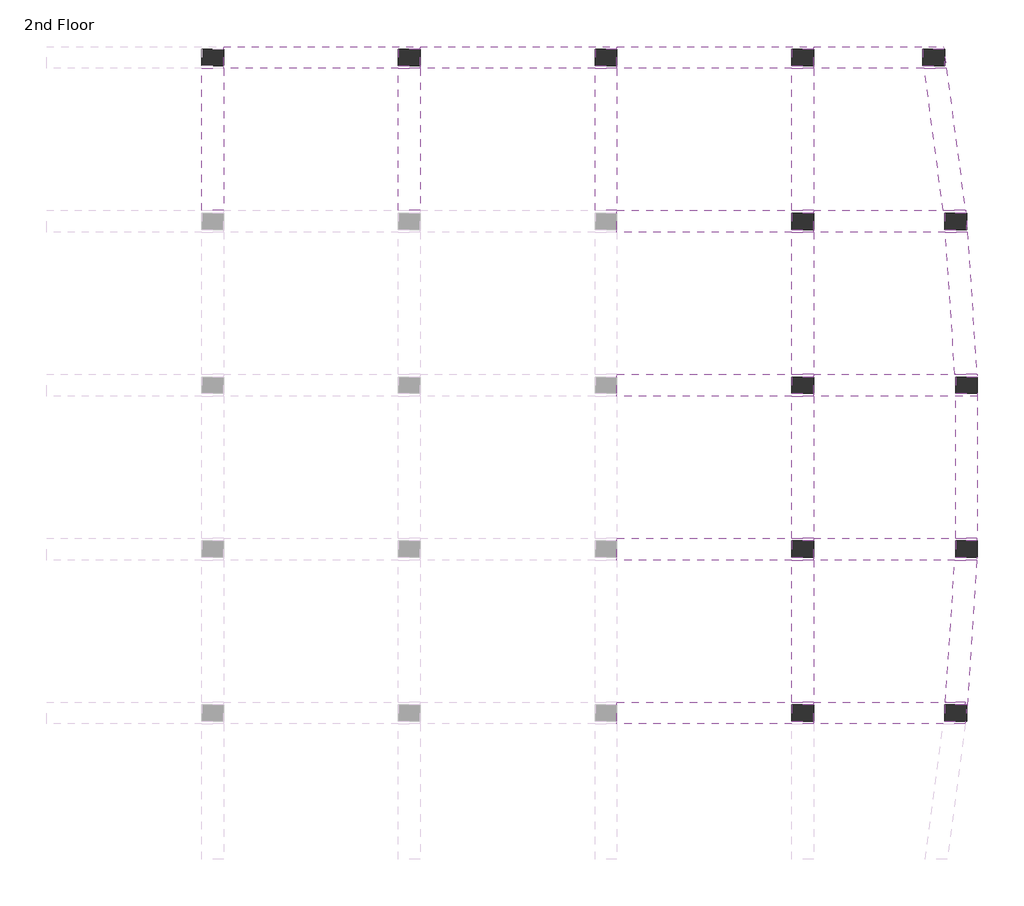
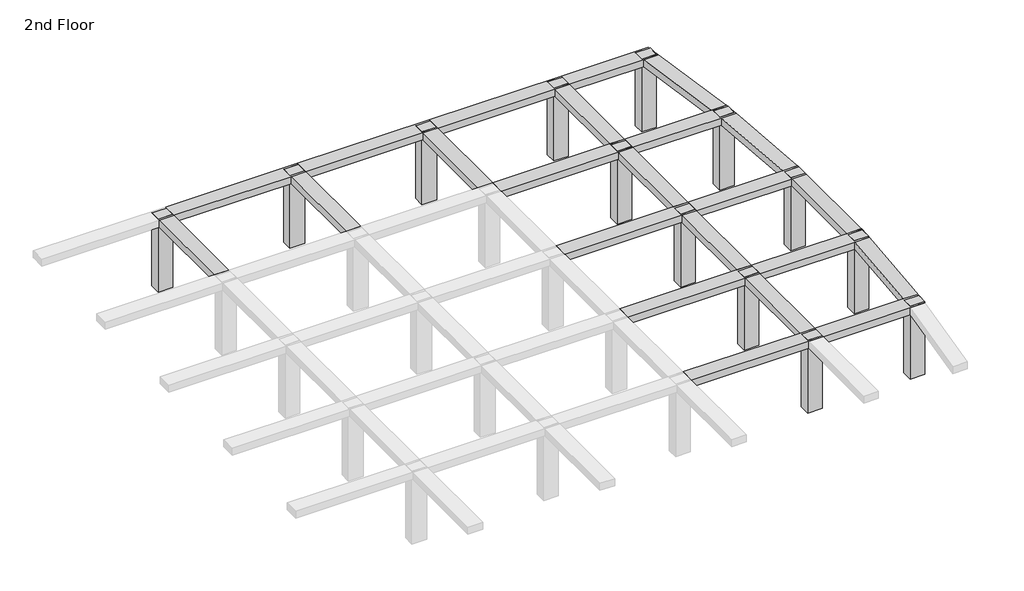
# One storey, part 3 of 3: 23 beams, 13 columns.
"""IFC4 building model written with IfcOpenShell, lengths in millimetres."""

from ifc_helpers import new_model, si_unit, frame, origin, place, context, project, spatial, polyline, outline, extrude, faceted_brep, element, save

model = new_model("IFC4")

# Units and contexts
model_context = context("Model", 3, world=origin())
ifc_project = project(units=[si_unit("LENGTHUNIT", "METRE", prefix="MILLI")], contexts=[model_context])

# Site, building, storey
site = spatial("IfcSite", under=ifc_project)
building = spatial("IfcBuilding", under=site)
storey = spatial("IfcBuildingStorey", under=building, Name="2nd Floor", Elevation=6400.8)

# Beams
placement = place(None, origin())
element("IfcBeam", 1, ObjectType="Concrete-Rectangular Beam : 2' x2'", at=placement, inside=storey, context=model_context, shape_type="Brep", body=[
    faceted_brep([(-160.074232, 1680.7831222, 9601.2), (-160.074232, 1604.5831222, 9601.2), (-160.074232, 1147.3831222, 9601.2), (-160.074232, 1071.1831222, 9601.2), (4716.725768, 1071.1831222, 9601.2), (5326.325768, 1071.1831222, 9601.2), (5326.325768, 1147.3831222, 9601.2), (4716.725768, 1147.3831222, 9601.2), (4716.725768, 1604.5831222, 9601.2), (5326.325768, 1604.5831222, 9601.2), (5326.325768, 1680.7831222, 9601.2), (4716.725768, 1680.7831222, 9601.2), (-160.074232, 1071.1831222, 9296.4), (4716.725768, 1071.1831222, 9296.4), (5326.325768, 1071.1831222, 9296.4), (-160.074232, 1147.3831222, 9296.4), (-160.074232, 1604.5831222, 9296.4), (-160.074232, 1680.7831222, 9296.4), (4716.725768, 1680.7831222, 9296.4), (5326.325768, 1680.7831222, 9296.4), (5326.325768, 1604.5831222, 9296.4), (4716.725768, 1604.5831222, 9296.4), (4716.725768, 1147.3831222, 9296.4), (5326.325768, 1147.3831222, 9296.4)], [[[0, 1, 2, 3, 4, 5, 6, 7, 8, 9, 10, 11]], [[3, 12, 13, 14, 5, 4]], [[12, 15, 16, 17, 18, 19, 20, 21, 22, 23, 14, 13]], [[10, 19, 18, 17, 0, 11]], [[3, 2, 1, 0, 17, 16, 15, 12]], [[5, 14, 23, 6]], [[22, 7, 6, 23]], [[7, 22, 21, 8]], [[8, 21, 20, 9]], [[19, 10, 9, 20]]]),
])
element("IfcBeam", 2, ObjectType="Concrete-Rectangular Beam : 2' x2'", at=placement, inside=storey, context=model_context, shape_type="Brep", body=[
    faceted_brep([(9555.2251658, 1680.7831222, 9601.2), (9003.0522312, 1680.7831222, 9601.2), (5326.325768, 1680.7831222, 9601.2), (5326.325768, 1604.5831222, 9601.2), (5326.325768, 1147.3831222, 9601.2), (5326.325768, 1071.1831222, 9601.2), (8940.2370643, 1071.1831222, 9601.2), (9555.2251658, 1071.1831222, 9601.2), (9555.2251658, 1147.3831222, 9601.2), (8983.5457827, 1147.3831222, 9601.2), (8983.5457827, 1604.5831222, 9601.2), (9555.2251658, 1604.5831222, 9601.2), (9555.2251658, 1071.1831222, 9296.4), (5326.325768, 1071.1831222, 9296.4), (8940.2370643, 1071.1831222, 9296.4), (5326.325768, 1147.3831222, 9296.4), (5326.325768, 1604.5831222, 9296.4), (5326.325768, 1680.7831222, 9296.4), (9003.0522312, 1680.7831222, 9296.4), (9555.2251658, 1680.7831222, 9296.4), (9555.2251658, 1604.5831222, 9296.4), (8983.5457827, 1604.5831222, 9296.4), (8983.5457827, 1147.3831222, 9296.4), (9555.2251658, 1147.3831222, 9296.4)], [[[0, 1, 2, 3, 4, 5, 6, 7, 8, 9, 10, 11]], [[12, 7, 6, 5, 13, 14]], [[12, 14, 13, 15, 16, 17, 18, 19, 20, 21, 22, 23]], [[0, 19, 18, 17, 2, 1]], [[7, 12, 23, 8]], [[5, 4, 3, 2, 17, 16, 15, 13]], [[22, 9, 8, 23]], [[9, 22, 21, 10]], [[10, 21, 20, 11]], [[19, 0, 11, 20]]]),
])
element("IfcBeam", 3, ObjectType="Concrete-Rectangular Beam : 2' x2'", at=placement, inside=storey, context=model_context, shape_type="Brep", body=[
    faceted_brep([(-160.074232, 6252.7831222, 9601.2), (-160.074232, 6176.5831222, 9601.2), (-160.074232, 5719.3831222, 9601.2), (-160.074232, 5643.1831222, 9601.2), (4716.725768, 5643.1831222, 9601.2), (5326.325768, 5643.1831222, 9601.2), (5326.325768, 5719.3831222, 9601.2), (4716.725768, 5719.3831222, 9601.2), (4716.725768, 6176.5831222, 9601.2), (5326.325768, 6176.5831222, 9601.2), (5326.325768, 6252.7831222, 9601.2), (4716.725768, 6252.7831222, 9601.2), (-160.074232, 5643.1831222, 9296.4), (4716.725768, 5643.1831222, 9296.4), (5326.325768, 5643.1831222, 9296.4), (-160.074232, 5719.3831222, 9296.4), (-160.074232, 6176.5831222, 9296.4), (-160.074232, 6252.7831222, 9296.4), (4716.725768, 6252.7831222, 9296.4), (5326.325768, 6252.7831222, 9296.4), (5326.325768, 6176.5831222, 9296.4), (4716.725768, 6176.5831222, 9296.4), (4716.725768, 5719.3831222, 9296.4), (5326.325768, 5719.3831222, 9296.4)], [[[0, 1, 2, 3, 4, 5, 6, 7, 8, 9, 10, 11]], [[3, 12, 13, 14, 5, 4]], [[12, 15, 16, 17, 18, 19, 20, 21, 22, 23, 14, 13]], [[10, 19, 18, 17, 0, 11]], [[3, 2, 1, 0, 17, 16, 15, 12]], [[5, 14, 23, 6]], [[22, 7, 6, 23]], [[7, 22, 21, 8]], [[8, 21, 20, 9]], [[19, 10, 9, 20]]]),
])
element("IfcBeam", 4, ObjectType="Concrete-Rectangular Beam : 2' x2'", at=placement, inside=storey, context=model_context, shape_type="Brep", body=[
    faceted_brep([(9876.2389574, 6252.7831222, 9601.2), (9286.1454059, 6252.7831222, 9601.2), (5326.325768, 6252.7831222, 9601.2), (5326.325768, 6176.5831222, 9601.2), (5326.325768, 5719.3831222, 9601.2), (5326.325768, 5643.1831222, 9601.2), (9265.305238, 5643.1831222, 9601.2), (9876.2389574, 5643.1831222, 9601.2), (9876.2389574, 5719.3831222, 9601.2), (9286.1454059, 5719.3831222, 9601.2), (9286.1454059, 6176.5831222, 9601.2), (9876.2389574, 6176.5831222, 9601.2), (9876.2389574, 5643.1831222, 9296.4), (5326.325768, 5643.1831222, 9296.4), (9265.305238, 5643.1831222, 9296.4), (5326.325768, 5719.3831222, 9296.4), (5326.325768, 6176.5831222, 9296.4), (5326.325768, 6252.7831222, 9296.4), (9286.1454059, 6252.7831222, 9296.4), (9876.2389574, 6252.7831222, 9296.4), (9876.2389574, 6176.5831222, 9296.4), (9286.1454059, 6176.5831222, 9296.4), (9286.1454059, 5719.3831222, 9296.4), (9876.2389574, 5719.3831222, 9296.4)], [[[0, 1, 2, 3, 4, 5, 6, 7, 8, 9, 10, 11]], [[12, 7, 6, 5, 13, 14]], [[12, 14, 13, 15, 16, 17, 18, 19, 20, 21, 22, 23]], [[0, 19, 18, 17, 2, 1]], [[7, 12, 23, 8]], [[5, 4, 3, 2, 17, 16, 15, 13]], [[22, 9, 8, 23]], [[9, 22, 21, 10]], [[10, 21, 20, 11]], [[19, 0, 11, 20]]]),
])
element("IfcBeam", 5, ObjectType="Concrete-Rectangular Beam : 2' x2'", at=placement, inside=storey, context=model_context, shape_type="Brep", body=[
    faceted_brep([(-160.074232, 10824.7831222, 9601.2), (-160.074232, 10748.5831222, 9601.2), (-160.074232, 10291.3831222, 9601.2), (-160.074232, 10215.1831222, 9601.2), (4716.725768, 10215.1831222, 9601.2), (5326.325768, 10215.1831222, 9601.2), (5326.325768, 10291.3831222, 9601.2), (4716.725768, 10291.3831222, 9601.2), (4716.725768, 10748.5831222, 9601.2), (5326.325768, 10748.5831222, 9601.2), (5326.325768, 10824.7831222, 9601.2), (4716.725768, 10824.7831222, 9601.2), (-160.074232, 10215.1831222, 9296.4), (4716.725768, 10215.1831222, 9296.4), (5326.325768, 10215.1831222, 9296.4), (-160.074232, 10291.3831222, 9296.4), (-160.074232, 10748.5831222, 9296.4), (-160.074232, 10824.7831222, 9296.4), (4716.725768, 10824.7831222, 9296.4), (5326.325768, 10824.7831222, 9296.4), (5326.325768, 10748.5831222, 9296.4), (4716.725768, 10748.5831222, 9296.4), (4716.725768, 10291.3831222, 9296.4), (5326.325768, 10291.3831222, 9296.4)], [[[0, 1, 2, 3, 4, 5, 6, 7, 8, 9, 10, 11]], [[3, 12, 13, 14, 5, 4]], [[12, 15, 16, 17, 18, 19, 20, 21, 22, 23, 14, 13]], [[10, 19, 18, 17, 0, 11]], [[3, 2, 1, 0, 17, 16, 15, 12]], [[5, 14, 23, 6]], [[22, 7, 6, 23]], [[7, 22, 21, 8]], [[8, 21, 20, 9]], [[19, 10, 9, 20]]]),
])
element("IfcBeam", 6, ObjectType="Concrete-Rectangular Beam : 2' x2'", at=placement, inside=storey, context=model_context, shape_type="Brep", body=[
    faceted_brep([(9895.7454059, 10824.7831222, 9601.2), (9876.2389574, 10824.7831222, 9601.2), (9265.305238, 10824.7831222, 9601.2), (5326.325768, 10824.7831222, 9601.2), (5326.325768, 10748.5831222, 9601.2), (5326.325768, 10291.3831222, 9601.2), (5326.325768, 10215.1831222, 9601.2), (9895.7454059, 10215.1831222, 9601.2), (9895.7454059, 10291.3831222, 9601.2), (9286.1454059, 10291.3831222, 9601.2), (9286.1454059, 10748.5831222, 9601.2), (9895.7454059, 10748.5831222, 9601.2), (9895.7454059, 10215.1831222, 9296.4), (5326.325768, 10215.1831222, 9296.4), (5326.325768, 10291.3831222, 9296.4), (5326.325768, 10748.5831222, 9296.4), (5326.325768, 10824.7831222, 9296.4), (9265.305238, 10824.7831222, 9296.4), (9876.2389574, 10824.7831222, 9296.4), (9895.7454059, 10824.7831222, 9296.4), (9895.7454059, 10748.5831222, 9296.4), (9286.1454059, 10748.5831222, 9296.4), (9286.1454059, 10291.3831222, 9296.4), (9895.7454059, 10291.3831222, 9296.4)], [[[0, 1, 2, 3, 4, 5, 6, 7, 8, 9, 10, 11]], [[12, 7, 6, 13]], [[12, 13, 14, 15, 16, 17, 18, 19, 20, 21, 22, 23]], [[0, 19, 18, 17, 16, 3, 2, 1]], [[7, 12, 23, 8]], [[6, 5, 4, 3, 16, 15, 14, 13]], [[22, 9, 8, 23]], [[9, 22, 21, 10]], [[10, 21, 20, 11]], [[19, 0, 11, 20]]]),
])
element("IfcBeam", 7, ObjectType="Concrete-Rectangular Beam : 2' x2'", at=placement, inside=storey, context=model_context, shape_type="Brep", body=[
    faceted_brep([(-160.074232, 15396.7831222, 9601.2), (-160.074232, 15320.5831222, 9601.2), (-160.074232, 14863.3831222, 9601.2), (-160.074232, 14787.1831222, 9601.2), (4716.725768, 14787.1831222, 9601.2), (5326.325768, 14787.1831222, 9601.2), (5326.325768, 14863.3831222, 9601.2), (4716.725768, 14863.3831222, 9601.2), (4716.725768, 15320.5831222, 9601.2), (5326.325768, 15320.5831222, 9601.2), (5326.325768, 15396.7831222, 9601.2), (4716.725768, 15396.7831222, 9601.2), (-160.074232, 14787.1831222, 9296.4), (4716.725768, 14787.1831222, 9296.4), (5326.325768, 14787.1831222, 9296.4), (-160.074232, 14863.3831222, 9296.4), (-160.074232, 15320.5831222, 9296.4), (-160.074232, 15396.7831222, 9296.4), (4716.725768, 15396.7831222, 9296.4), (5326.325768, 15396.7831222, 9296.4), (5326.325768, 15320.5831222, 9296.4), (4716.725768, 15320.5831222, 9296.4), (4716.725768, 14863.3831222, 9296.4), (5326.325768, 14863.3831222, 9296.4)], [[[0, 1, 2, 3, 4, 5, 6, 7, 8, 9, 10, 11]], [[3, 12, 13, 14, 5, 4]], [[12, 15, 16, 17, 18, 19, 20, 21, 22, 23, 14, 13]], [[10, 19, 18, 17, 0, 11]], [[3, 2, 1, 0, 17, 16, 15, 12]], [[5, 14, 23, 6]], [[22, 7, 6, 23]], [[7, 22, 21, 8]], [[8, 21, 20, 9]], [[19, 10, 9, 20]]]),
])
element("IfcBeam", 8, ObjectType="Concrete-Rectangular Beam : 2' x2'", at=placement, inside=storey, context=model_context, shape_type="Brep", body=[
    faceted_brep([(9573.6393342, 15396.7831222, 9601.2), (9555.2251658, 15396.7831222, 9601.2), (8940.2370643, 15396.7831222, 9601.2), (5326.325768, 15396.7831222, 9601.2), (5326.325768, 15320.5831222, 9601.2), (5326.325768, 14863.3831222, 9601.2), (5326.325768, 14787.1831222, 9601.2), (9003.0522312, 14787.1831222, 9601.2), (9613.9859506, 14787.1831222, 9601.2), (9593.1457827, 15102.0587543, 9601.2), (9593.1457827, 14863.3831222, 9601.2), (8983.5457827, 14863.3831222, 9601.2), (8983.5457827, 15320.5831222, 9601.2), (9578.6826612, 15320.5831222, 9601.2), (9613.9859506, 14787.1831222, 9296.4), (5326.325768, 14787.1831222, 9296.4), (9003.0522312, 14787.1831222, 9296.4), (5326.325768, 14863.3831222, 9296.4), (5326.325768, 15320.5831222, 9296.4), (5326.325768, 15396.7831222, 9296.4), (8940.2370643, 15396.7831222, 9296.4), (9555.2251658, 15396.7831222, 9296.4), (9573.6393342, 15396.7831222, 9296.4), (9578.6826612, 15320.5831222, 9296.4), (8983.5457827, 15320.5831222, 9296.4), (8983.5457827, 14863.3831222, 9296.4), (9593.1457827, 14863.3831222, 9296.4), (9593.1457827, 15102.0587543, 9296.4)], [[[0, 1, 2, 3, 4, 5, 6, 7, 8, 9, 10, 11, 12, 13]], [[14, 8, 7, 6, 15, 16]], [[14, 16, 15, 17, 18, 19, 20, 21, 22, 23, 24, 25, 26, 27]], [[0, 22, 21, 20, 19, 3, 2, 1]], [[8, 14, 27, 9]], [[6, 5, 4, 3, 19, 18, 17, 15]], [[26, 10, 9, 27]], [[10, 26, 25, 11]], [[11, 25, 24, 12]], [[12, 24, 23, 13]], [[22, 0, 13, 23]]]),
])
element("IfcBeam", 9, ObjectType="Concrete-Rectangular Beam : 2' x2'", at=placement, inside=storey, context=model_context, shape_type="Brep", body=[
    faceted_brep([(-11132.874232, 19968.7831222, 9601.2), (-11132.874232, 19892.5831222, 9601.2), (-11132.874232, 19435.3831222, 9601.2), (-11132.874232, 19359.1831222, 9601.2), (-6256.074232, 19359.1831222, 9601.2), (-5646.474232, 19359.1831222, 9601.2), (-5646.474232, 19435.3831222, 9601.2), (-6256.074232, 19435.3831222, 9601.2), (-6256.074232, 19892.5831222, 9601.2), (-5646.474232, 19892.5831222, 9601.2), (-5646.474232, 19968.7831222, 9601.2), (-11132.874232, 19359.1831222, 9296.4), (-6256.074232, 19359.1831222, 9296.4), (-5646.474232, 19359.1831222, 9296.4), (-11132.874232, 19435.3831222, 9296.4), (-11132.874232, 19892.5831222, 9296.4), (-11132.874232, 19968.7831222, 9296.4), (-5646.474232, 19968.7831222, 9296.4), (-5646.474232, 19892.5831222, 9296.4), (-6256.074232, 19892.5831222, 9296.4), (-6256.074232, 19435.3831222, 9296.4), (-5646.474232, 19435.3831222, 9296.4)], [[[0, 1, 2, 3, 4, 5, 6, 7, 8, 9, 10]], [[3, 11, 12, 13, 5, 4]], [[11, 14, 15, 16, 17, 18, 19, 20, 21, 13, 12]], [[10, 17, 16, 0]], [[3, 2, 1, 0, 16, 15, 14, 11]], [[5, 13, 21, 6]], [[20, 7, 6, 21]], [[7, 20, 19, 8]], [[8, 19, 18, 9]], [[17, 10, 9, 18]]]),
])
element("IfcBeam", 10, ObjectType="Concrete-Rectangular Beam : 2' x2'", at=placement, inside=storey, context=model_context, shape_type="Brep", body=[
    faceted_brep([(-160.074232, 19968.7831222, 9601.2), (-5646.474232, 19968.7831222, 9601.2), (-5646.474232, 19892.5831222, 9601.2), (-5646.474232, 19435.3831222, 9601.2), (-5646.474232, 19359.1831222, 9601.2), (-769.674232, 19359.1831222, 9601.2), (-160.074232, 19359.1831222, 9601.2), (-160.074232, 19435.3831222, 9601.2), (-769.674232, 19435.3831222, 9601.2), (-769.674232, 19892.5831222, 9601.2), (-160.074232, 19892.5831222, 9601.2), (-160.074232, 19359.1831222, 9296.4), (-5646.474232, 19359.1831222, 9296.4), (-769.674232, 19359.1831222, 9296.4), (-5646.474232, 19435.3831222, 9296.4), (-5646.474232, 19892.5831222, 9296.4), (-5646.474232, 19968.7831222, 9296.4), (-160.074232, 19968.7831222, 9296.4), (-160.074232, 19892.5831222, 9296.4), (-769.674232, 19892.5831222, 9296.4), (-769.674232, 19435.3831222, 9296.4), (-160.074232, 19435.3831222, 9296.4)], [[[0, 1, 2, 3, 4, 5, 6, 7, 8, 9, 10]], [[11, 6, 5, 4, 12, 13]], [[11, 13, 12, 14, 15, 16, 17, 18, 19, 20, 21]], [[0, 17, 16, 1]], [[6, 11, 21, 7]], [[4, 3, 2, 1, 16, 15, 14, 12]], [[20, 8, 7, 21]], [[8, 20, 19, 9]], [[9, 19, 18, 10]], [[17, 0, 10, 18]]]),
])
element("IfcBeam", 11, ObjectType="Concrete-Rectangular Beam : 2' x2'", at=placement, inside=storey, context=model_context, shape_type="Brep", body=[
    faceted_brep([(-160.074232, 19968.7831222, 9601.2), (-160.074232, 19892.5831222, 9601.2), (-160.074232, 19435.3831222, 9601.2), (-160.074232, 19359.1831222, 9601.2), (4716.725768, 19359.1831222, 9601.2), (5326.325768, 19359.1831222, 9601.2), (5326.325768, 19435.3831222, 9601.2), (4716.725768, 19435.3831222, 9601.2), (4716.725768, 19892.5831222, 9601.2), (5326.325768, 19892.5831222, 9601.2), (5326.325768, 19968.7831222, 9601.2), (-160.074232, 19359.1831222, 9296.4), (4716.725768, 19359.1831222, 9296.4), (5326.325768, 19359.1831222, 9296.4), (-160.074232, 19435.3831222, 9296.4), (-160.074232, 19892.5831222, 9296.4), (-160.074232, 19968.7831222, 9296.4), (5326.325768, 19968.7831222, 9296.4), (5326.325768, 19892.5831222, 9296.4), (4716.725768, 19892.5831222, 9296.4), (4716.725768, 19435.3831222, 9296.4), (5326.325768, 19435.3831222, 9296.4)], [[[0, 1, 2, 3, 4, 5, 6, 7, 8, 9, 10]], [[3, 11, 12, 13, 5, 4]], [[11, 14, 15, 16, 17, 18, 19, 20, 21, 13, 12]], [[10, 17, 16, 0]], [[3, 2, 1, 0, 16, 15, 14, 11]], [[5, 13, 21, 6]], [[20, 7, 6, 21]], [[7, 20, 19, 8]], [[8, 19, 18, 9]], [[17, 10, 9, 18]]]),
])
element("IfcBeam", 12, ObjectType="Concrete-Rectangular Beam : 2' x2'", at=placement, inside=storey, context=model_context, shape_type="Brep", body=[
    faceted_brep([(5326.325768, 19968.7831222, 9601.2), (5326.325768, 19892.5831222, 9601.2), (5326.325768, 19435.3831222, 9601.2), (5326.325768, 19359.1831222, 9601.2), (8412.2463849, 19359.1831222, 9601.2), (9027.2344863, 19359.1831222, 9601.2), (8983.925768, 19684.2011052, 9601.2), (8983.925768, 19435.3831222, 9601.2), (8374.325768, 19435.3831222, 9601.2), (8374.325768, 19892.5831222, 9601.2), (8956.158818, 19892.5831222, 9601.2), (8946.005151, 19968.7831222, 9601.2), (5326.325768, 19359.1831222, 9296.4), (8412.2463849, 19359.1831222, 9296.4), (9027.2344863, 19359.1831222, 9296.4), (5326.325768, 19435.3831222, 9296.4), (5326.325768, 19892.5831222, 9296.4), (5326.325768, 19968.7831222, 9296.4), (8946.005151, 19968.7831222, 9296.4), (8956.158818, 19892.5831222, 9296.4), (8374.325768, 19892.5831222, 9296.4), (8374.325768, 19435.3831222, 9296.4), (8983.925768, 19435.3831222, 9296.4), (8983.925768, 19684.2011052, 9296.4)], [[[0, 1, 2, 3, 4, 5, 6, 7, 8, 9, 10, 11]], [[3, 12, 13, 14, 5, 4]], [[12, 15, 16, 17, 18, 19, 20, 21, 22, 23, 14, 13]], [[11, 18, 17, 0]], [[3, 2, 1, 0, 17, 16, 15, 12]], [[5, 14, 23, 6]], [[22, 7, 6, 23]], [[7, 22, 21, 8]], [[8, 21, 20, 9]], [[9, 20, 19, 10]], [[18, 11, 10, 19]]]),
])
element("IfcBeam", 13, ObjectType="Concrete-Rectangular Beam : 2' x2'", at=placement, inside=storey, context=model_context, shape_type="SweptSolid", body=[
    extrude(outline(polyline([(-11132.874232, 15396.7831222), (-11742.474232, 15396.7831222), (-11742.474232, 19359.1831222), (-11132.874232, 19359.1831222), (-11132.874232, 15396.7831222)])), frame((0.0, 0.0, 9296.4), z_axis=(0.0, 0.0, 1.0), x_axis=(1.0, 0.0, 0.0)), (0.0, 0.0, 1.0), 304.8),
])
element("IfcBeam", 14, ObjectType="Concrete-Rectangular Beam : 2' x2'", at=placement, inside=storey, context=model_context, shape_type="SweptSolid", body=[
    extrude(outline(polyline([(-5646.474232, 15396.7831222), (-6256.074232, 15396.7831222), (-6256.074232, 19359.1831222), (-5646.474232, 19359.1831222), (-5646.474232, 15396.7831222)])), frame((0.0, 0.0, 9296.4), z_axis=(0.0, 0.0, 1.0), x_axis=(1.0, 0.0, 0.0)), (0.0, 0.0, 1.0), 304.8),
])
element("IfcBeam", 15, ObjectType="Concrete-Rectangular Beam : 2' x2'", at=placement, inside=storey, context=model_context, shape_type="SweptSolid", body=[
    extrude(outline(polyline([(-160.074232, 15396.7831222), (-769.674232, 15396.7831222), (-769.674232, 19359.1831222), (-160.074232, 19359.1831222), (-160.074232, 15396.7831222)])), frame((0.0, 0.0, 9296.4), z_axis=(0.0, 0.0, 1.0), x_axis=(1.0, 0.0, 0.0)), (0.0, 0.0, 1.0), 304.8),
])
element("IfcBeam", 16, ObjectType="Concrete-Rectangular Beam : 2' x2'", at=placement, inside=storey, context=model_context, shape_type="SweptSolid", body=[
    extrude(outline(polyline([(5326.325768, 1680.7831222), (4716.725768, 1680.7831222), (4716.725768, 5643.1831222), (5326.325768, 5643.1831222), (5326.325768, 1680.7831222)])), frame((0.0, 0.0, 9296.4), z_axis=(0.0, 0.0, 1.0), x_axis=(1.0, 0.0, 0.0)), (0.0, 0.0, 1.0), 304.8),
])
element("IfcBeam", 17, ObjectType="Concrete-Rectangular Beam : 2' x2'", at=placement, inside=storey, context=model_context, shape_type="SweptSolid", body=[
    extrude(outline(polyline([(4716.725768, 10215.1831222), (5326.325768, 10215.1831222), (5326.325768, 6252.7831222), (4716.725768, 6252.7831222), (4716.725768, 10215.1831222)])), frame((0.0, 0.0, 9296.4), z_axis=(0.0, 0.0, 1.0), x_axis=(1.0, 0.0, 0.0)), (0.0, 0.0, 1.0), 304.8),
])
element("IfcBeam", 18, ObjectType="Concrete-Rectangular Beam : 2' x2'", at=placement, inside=storey, context=model_context, shape_type="SweptSolid", body=[
    extrude(outline(polyline([(4716.725768, 14787.1831222), (5326.325768, 14787.1831222), (5326.325768, 10824.7831222), (4716.725768, 10824.7831222), (4716.725768, 14787.1831222)])), frame((0.0, 0.0, 9296.4), z_axis=(0.0, 0.0, 1.0), x_axis=(1.0, 0.0, 0.0)), (0.0, 0.0, 1.0), 304.8),
])
element("IfcBeam", 19, ObjectType="Concrete-Rectangular Beam : 2' x2'", at=placement, inside=storey, context=model_context, shape_type="SweptSolid", body=[
    extrude(outline(polyline([(5326.325768, 15396.7831222), (4716.725768, 15396.7831222), (4716.725768, 19359.1831222), (5326.325768, 19359.1831222), (5326.325768, 15396.7831222)])), frame((0.0, 0.0, 9296.4), z_axis=(0.0, 0.0, 1.0), x_axis=(1.0, 0.0, 0.0)), (0.0, 0.0, 1.0), 304.8),
])
element("IfcBeam", 20, ObjectType="Concrete-Rectangular Beam : 2' x2'", at=placement, inside=storey, context=model_context, shape_type="Brep", body=[
    faceted_brep([(9916.5855738, 6252.7831222, 9601.2), (9895.7454059, 6252.7831222, 9601.2), (9876.2389574, 6252.7831222, 9601.2), (9876.2389574, 6176.5831222, 9601.2), (9895.7454059, 6176.5831222, 9601.2), (9895.7454059, 5937.9074901, 9601.2), (9916.5855738, 6252.7831222, 9296.4), (9895.7454059, 5937.9074901, 9296.4), (9876.2389574, 6252.7831222, 9296.4), (9895.7454059, 6252.7831222, 9296.4), (9895.7454059, 6176.5831222, 9296.4), (9876.2389574, 6176.5831222, 9296.4)], [[[0, 1, 2, 3, 4, 5]], [[6, 0, 5, 7]], [[8, 9, 6, 7, 10, 11]], [[0, 6, 9, 8, 2, 1]], [[4, 10, 7, 5]], [[10, 4, 3, 11]], [[2, 8, 11, 3]]]),
    faceted_brep([(9003.0522312, 1680.7831222, 9296.4), (9003.0522312, 1680.7831222, 9601.2), (9265.305238, 5643.1831222, 9601.2), (9265.305238, 5643.1831222, 9296.4), (9021.4663996, 1680.7831222, 9296.4), (9555.2251658, 1680.7831222, 9296.4), (9555.2251658, 1680.7831222, 9601.2), (9021.4663996, 1680.7831222, 9601.2), (9876.2389574, 5643.1831222, 9601.2), (9876.2389574, 5643.1831222, 9296.4), (9876.2389574, 5719.3831222, 9601.2), (9876.2389574, 5719.3831222, 9296.4), (9555.2251658, 1604.5831222, 9601.2), (9593.1457827, 1604.5831222, 9601.2), (9593.1457827, 1365.9074901, 9601.2), (9593.1457827, 1365.9074901, 9296.4), (9593.1457827, 1604.5831222, 9296.4), (9555.2251658, 1604.5831222, 9296.4), (9881.2822845, 5719.3831222, 9601.2), (9881.2822845, 5719.3831222, 9296.4)], [[[0, 1, 2, 3]], [[1, 0, 4, 5, 6, 7]], [[2, 8, 9, 3]], [[9, 8, 10, 11]], [[8, 2, 1, 7, 6, 12, 13, 14]], [[3, 9, 15, 16, 17, 5, 4, 0]], [[13, 16, 15, 14]], [[16, 13, 12, 17]], [[6, 5, 17, 12]], [[10, 18, 19, 11]], [[10, 8, 18]], [[8, 14, 15, 9, 19, 18]], [[19, 9, 11]]]),
    faceted_brep([(9555.2251658, 1071.1831222, 9601.2), (9555.2251658, 1071.1831222, 9296.4), (9565.3788327, 1147.3831222, 9296.4), (9565.3788327, 1147.3831222, 9601.2), (9555.2251658, 1147.3831222, 9601.2), (9555.2251658, 1147.3831222, 9296.4)], [[[0, 1, 2, 3]], [[1, 0, 4, 5]], [[3, 2, 5, 4]], [[4, 0, 3]], [[2, 1, 5]]]),
])
element("IfcBeam", 21, ObjectType="Concrete-Rectangular Beam : 2' x2'", at=placement, inside=storey, context=model_context, shape_type="Brep", body=[
    faceted_brep([(9895.7454059, 10824.7831222, 9601.2), (9876.2389574, 10824.7831222, 9601.2), (9286.1454059, 10824.7831222, 9601.2), (9286.1454059, 10748.5831222, 9601.2), (9895.7454059, 10748.5831222, 9601.2), (9895.7454059, 10824.7831222, 9296.4), (9895.7454059, 10748.5831222, 9296.4), (9286.1454059, 10824.7831222, 9296.4), (9876.2389574, 10824.7831222, 9296.4), (9286.1454059, 10748.5831222, 9296.4)], [[[0, 1, 2, 3, 4]], [[5, 0, 4, 6]], [[7, 8, 5, 6, 9]], [[2, 7, 9, 3]], [[2, 1, 0, 5, 8, 7]], [[4, 3, 9, 6]]]),
    faceted_brep([(9286.1454059, 6252.7831222, 9601.2), (9286.1454059, 6252.7831222, 9296.4), (9876.2389574, 6252.7831222, 9296.4), (9895.7454059, 6252.7831222, 9296.4), (9895.7454059, 6252.7831222, 9601.2), (9876.2389574, 6252.7831222, 9601.2), (9286.1454059, 10291.3831222, 9601.2), (9895.7454059, 10291.3831222, 9601.2), (9895.7454059, 10291.3831222, 9296.4), (9286.1454059, 10291.3831222, 9296.4)], [[[0, 1, 2, 3, 4, 5]], [[6, 7, 8, 9]], [[0, 5, 4, 7, 6]], [[4, 3, 8, 7]], [[3, 2, 1, 9, 8]], [[1, 0, 6, 9]]]),
])
element("IfcBeam", 22, ObjectType="Concrete-Rectangular Beam : 2' x2'", at=placement, inside=storey, context=model_context, shape_type="Brep", body=[
    faceted_brep([(9613.9859506, 14787.1831222, 9601.2), (9003.0522312, 14787.1831222, 9601.2), (9265.305238, 10824.7831222, 9601.2), (9286.1454059, 10824.7831222, 9601.2), (9876.2389574, 10824.7831222, 9601.2), (9613.9859506, 14787.1831222, 9296.4), (9876.2389574, 10824.7831222, 9296.4), (9003.0522312, 14787.1831222, 9296.4), (9286.1454059, 10824.7831222, 9296.4), (9265.305238, 10824.7831222, 9296.4)], [[[0, 1, 2, 3, 4]], [[5, 0, 4, 6]], [[7, 5, 6, 8, 9]], [[1, 7, 9, 2]], [[1, 0, 5, 7]], [[4, 3, 2, 9, 8, 6]]]),
])
element("IfcBeam", 23, ObjectType="Concrete-Rectangular Beam : 2' x2'", at=placement, inside=storey, context=model_context, shape_type="SweptSolid", body=[
    extrude(outline(polyline([(8412.2463849, 19359.1831222), (9027.2344863, 19359.1831222), (9555.2251658, 15396.7831222), (8940.2370643, 15396.7831222), (8412.2463849, 19359.1831222)])), frame((0.0, 0.0, 9296.4), z_axis=(0.0, 0.0, 1.0), x_axis=(1.0, 0.0, 0.0)), (0.0, 0.0, 1.0), 304.8),
])

# Columns
element("IfcColumn", 24, ObjectType="Concrete-Rectangular-Column : 12 x 18", at=placement, inside=storey, context=model_context, shape_type="SweptSolid", body=[
    extrude(outline(polyline([(5326.325768, 1604.5831222), (5326.325768, 1147.3831222), (4716.725768, 1147.3831222), (4716.725768, 1604.5831222), (5326.325768, 1604.5831222)])), frame((0.0, 0.0, 6400.8), z_axis=(0.0, 0.0, 1.0), x_axis=(1.0, 0.0, 0.0)), (0.0, 0.0, 1.0), 3200.4),
])
element("IfcColumn", 25, ObjectType="Concrete-Rectangular-Column : 12 x 18", at=placement, inside=storey, context=model_context, shape_type="SweptSolid", body=[
    extrude(outline(polyline([(9593.1457827, 1604.5831222), (9593.1457827, 1147.3831222), (8983.5457827, 1147.3831222), (8983.5457827, 1604.5831222), (9593.1457827, 1604.5831222)])), frame((0.0, 0.0, 6400.8), z_axis=(0.0, 0.0, 1.0), x_axis=(1.0, 0.0, 0.0)), (0.0, 0.0, 1.0), 3200.4),
])
element("IfcColumn", 26, ObjectType="Concrete-Rectangular-Column : 12 x 18", at=placement, inside=storey, context=model_context, shape_type="SweptSolid", body=[
    extrude(outline(polyline([(5326.325768, 6176.5831222), (5326.325768, 5719.3831222), (4716.725768, 5719.3831222), (4716.725768, 6176.5831222), (5326.325768, 6176.5831222)])), frame((0.0, 0.0, 6400.8), z_axis=(0.0, 0.0, 1.0), x_axis=(1.0, 0.0, 0.0)), (0.0, 0.0, 1.0), 3200.4),
])
element("IfcColumn", 27, ObjectType="Concrete-Rectangular-Column : 12 x 18", at=placement, inside=storey, context=model_context, shape_type="SweptSolid", body=[
    extrude(outline(polyline([(9895.7454059, 6176.5831222), (9895.7454059, 5719.3831222), (9286.1454059, 5719.3831222), (9286.1454059, 6176.5831222), (9895.7454059, 6176.5831222)])), frame((0.0, 0.0, 6400.8), z_axis=(0.0, 0.0, 1.0), x_axis=(1.0, 0.0, 0.0)), (0.0, 0.0, 1.0), 3200.4),
])
element("IfcColumn", 28, ObjectType="Concrete-Rectangular-Column : 12 x 18", at=placement, inside=storey, context=model_context, shape_type="SweptSolid", body=[
    extrude(outline(polyline([(5326.325768, 10748.5831222), (5326.325768, 10291.3831222), (4716.725768, 10291.3831222), (4716.725768, 10748.5831222), (5326.325768, 10748.5831222)])), frame((0.0, 0.0, 6400.8), z_axis=(0.0, 0.0, 1.0), x_axis=(1.0, 0.0, 0.0)), (0.0, 0.0, 1.0), 3200.4),
])
element("IfcColumn", 29, ObjectType="Concrete-Rectangular-Column : 12 x 18", at=placement, inside=storey, context=model_context, shape_type="SweptSolid", body=[
    extrude(outline(polyline([(9895.7454059, 10748.5831222), (9895.7454059, 10291.3831222), (9286.1454059, 10291.3831222), (9286.1454059, 10748.5831222), (9895.7454059, 10748.5831222)])), frame((0.0, 0.0, 6400.8), z_axis=(0.0, 0.0, 1.0), x_axis=(1.0, 0.0, 0.0)), (0.0, 0.0, 1.0), 3200.4),
])
element("IfcColumn", 30, ObjectType="Concrete-Rectangular-Column : 12 x 18", at=placement, inside=storey, context=model_context, shape_type="SweptSolid", body=[
    extrude(outline(polyline([(5326.325768, 15320.5831222), (5326.325768, 14863.3831222), (4716.725768, 14863.3831222), (4716.725768, 15320.5831222), (5326.325768, 15320.5831222)])), frame((0.0, 0.0, 6400.8), z_axis=(0.0, 0.0, 1.0), x_axis=(1.0, 0.0, 0.0)), (0.0, 0.0, 1.0), 3200.4),
])
element("IfcColumn", 31, ObjectType="Concrete-Rectangular-Column : 12 x 18", at=placement, inside=storey, context=model_context, shape_type="SweptSolid", body=[
    extrude(outline(polyline([(9593.1457827, 15320.5831222), (9593.1457827, 14863.3831222), (8983.5457827, 14863.3831222), (8983.5457827, 15320.5831222), (9593.1457827, 15320.5831222)])), frame((0.0, 0.0, 6400.8), z_axis=(0.0, 0.0, 1.0), x_axis=(1.0, 0.0, 0.0)), (0.0, 0.0, 1.0), 3200.4),
])
element("IfcColumn", 32, ObjectType="Concrete-Rectangular-Column : 12 x 18", at=placement, inside=storey, context=model_context, shape_type="SweptSolid", body=[
    extrude(outline(polyline([(-11132.874232, 19892.5831222), (-11132.874232, 19435.3831222), (-11742.474232, 19435.3831222), (-11742.474232, 19892.5831222), (-11132.874232, 19892.5831222)])), frame((0.0, 0.0, 6400.8), z_axis=(0.0, 0.0, 1.0), x_axis=(1.0, 0.0, 0.0)), (0.0, 0.0, 1.0), 3200.4),
])
element("IfcColumn", 33, ObjectType="Concrete-Rectangular-Column : 12 x 18", at=placement, inside=storey, context=model_context, shape_type="SweptSolid", body=[
    extrude(outline(polyline([(-5646.474232, 19892.5831222), (-5646.474232, 19435.3831222), (-6256.074232, 19435.3831222), (-6256.074232, 19892.5831222), (-5646.474232, 19892.5831222)])), frame((0.0, 0.0, 6400.8), z_axis=(0.0, 0.0, 1.0), x_axis=(1.0, 0.0, 0.0)), (0.0, 0.0, 1.0), 3200.4),
])
element("IfcColumn", 34, ObjectType="Concrete-Rectangular-Column : 12 x 18", at=placement, inside=storey, context=model_context, shape_type="SweptSolid", body=[
    extrude(outline(polyline([(-160.074232, 19892.5831222), (-160.074232, 19435.3831222), (-769.674232, 19435.3831222), (-769.674232, 19892.5831222), (-160.074232, 19892.5831222)])), frame((0.0, 0.0, 6400.8), z_axis=(0.0, 0.0, 1.0), x_axis=(1.0, 0.0, 0.0)), (0.0, 0.0, 1.0), 3200.4),
])
element("IfcColumn", 35, ObjectType="Concrete-Rectangular-Column : 12 x 18", at=placement, inside=storey, context=model_context, shape_type="SweptSolid", body=[
    extrude(outline(polyline([(5326.325768, 19892.5831222), (5326.325768, 19435.3831222), (4716.725768, 19435.3831222), (4716.725768, 19892.5831222), (5326.325768, 19892.5831222)])), frame((0.0, 0.0, 6400.8), z_axis=(0.0, 0.0, 1.0), x_axis=(1.0, 0.0, 0.0)), (0.0, 0.0, 1.0), 3200.4),
])
element("IfcColumn", 36, ObjectType="Concrete-Rectangular-Column : 12 x 18", at=placement, inside=storey, context=model_context, shape_type="SweptSolid", body=[
    extrude(outline(polyline([(8983.925768, 19892.5831222), (8983.925768, 19435.3831222), (8374.325768, 19435.3831222), (8374.325768, 19892.5831222), (8983.925768, 19892.5831222)])), frame((0.0, 0.0, 6400.8), z_axis=(0.0, 0.0, 1.0), x_axis=(1.0, 0.0, 0.0)), (0.0, 0.0, 1.0), 3200.4),
])

save(model, "model.ifc")

# Revit data of these elements
# Type "Concrete-Rectangular Beam : 2' x2'"
#   Assembly Code = "B10"
#   Length [instance default] = 5' - 0"
#   b = 2' - 0"
#   h = 1' - 0"
#   Structural Material [instance default] = Concrete, Cast-in-Place gray
# Type "Concrete-Rectangular-Column : 12 x 18"
#   Assembly Code = "B10"
#   b = 2' - 0"
#   h = 1' - 6"
#   Structural Material [instance default] = Concrete, Cast-in-Place gray
# Elements 1, 2, 3, 4, 5, 6, 7, 8, 9, 10, 11, 12, 13, 14, 15, 16, 17, 18, 19, 20, 21, 22, 23 (IfcBeam, "Concrete-Rectangular Beam : 2' x2'")
#   Structural Material = Concrete, Precast (2)
#   Phase Created = New Construction
#   Materials on its faces: "Concrete, Precast (2)"
# Elements 24, 25, 26, 27, 28, 29, 30, 31, 32, 33, 34, 35, 36 (IfcColumn, "Concrete-Rectangular-Column : 12 x 18")
#   Phase Created = New Construction
#   Materials on its faces: "Concrete, Cast-in-Place gray"
# Materials
#   "Concrete, Cast-in-Place gray": class "Concrete", colour RGB 192 192 192, transparency 0, Description = "Cast-in-place concrete", Cost = 0
#   "Concrete, Precast (2)": class "Concrete", colour RGB 198 187 187, transparency 0, Description = "Precast concrete", Cost = 0
